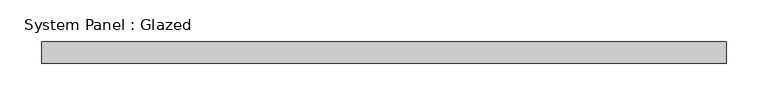
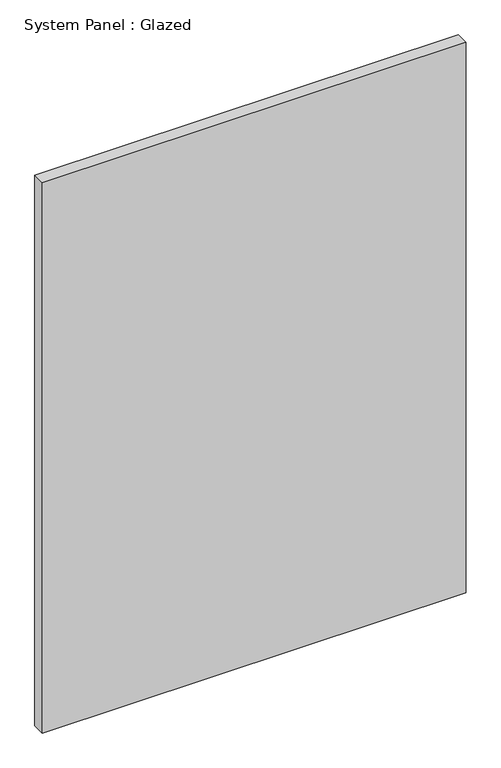
"""IFC4 building model written with IfcOpenShell, lengths in millimetres: plate geometry, System Panel : Glazed."""

from ifc_helpers import new_model, si_unit, origin, origin_with_axes, place, context, project, spatial, polyline, outline, extrude, source, transform, mapped, element, save


def system_panel_glazed_231200ce(model_context):
    return source(origin(), model_context, "Body", "SweptSolid", [
        extrude(outline(polyline([(409.575, 19.05), (-409.575, 19.05), (-409.575, 44.45), (409.575, 44.45), (409.575, 19.05)])), origin_with_axes(), (0.0, 0.0, 1.0), 1123.95),
    ])


if __name__ == "__main__":
    model = new_model("IFC4")
    model_context = context("Model", 3, world=origin())
    ifc_project = project(units=[si_unit("LENGTHUNIT", "METRE", prefix="MILLI")], contexts=[model_context])
    site = spatial("IfcSite", under=ifc_project)
    building = spatial("IfcBuilding", under=site)
    placement = place(None, origin())
    system_panel_glazed_shape = system_panel_glazed_231200ce(model_context)
    element("IfcPlate", 1, ObjectType="System Panel : Glazed", at=placement, inside=building, context=model_context, shape_type="MappedRepresentation", body=[
        mapped(system_panel_glazed_shape, transform((0.0, 0.0, 0.0), x_axis=(1.0, 0.0, 0.0), y_axis=(0.0, 1.0, 0.0), z_axis=(0.0, 0.0, 1.0))),
    ])
    save(model, "model.ifc")

# Revit data of these elements
# Type "System Panel : Glazed"
#   Construction Type Id = "GSP4R"
#   Analytic Construction = "1/8 in Pilkington single glazing"
#   Visual Light Transmittance = 0.9
#   Solar Heat Gain Coefficient = 0.86
#   Heat Transfer Coefficient (U) = 1.18115 BTU/(h·ft²·°F)
#   Define Thermal Properties by = 1
# Element 1 (IfcPlate, "System Panel : Glazed")
#   Materials on its faces: "Glass"
# Materials
#   "Glass": class "Glass", colour RGB 0 128 192, transparency 0.75, Description = "Soda Lime Glass", Cost = 0
